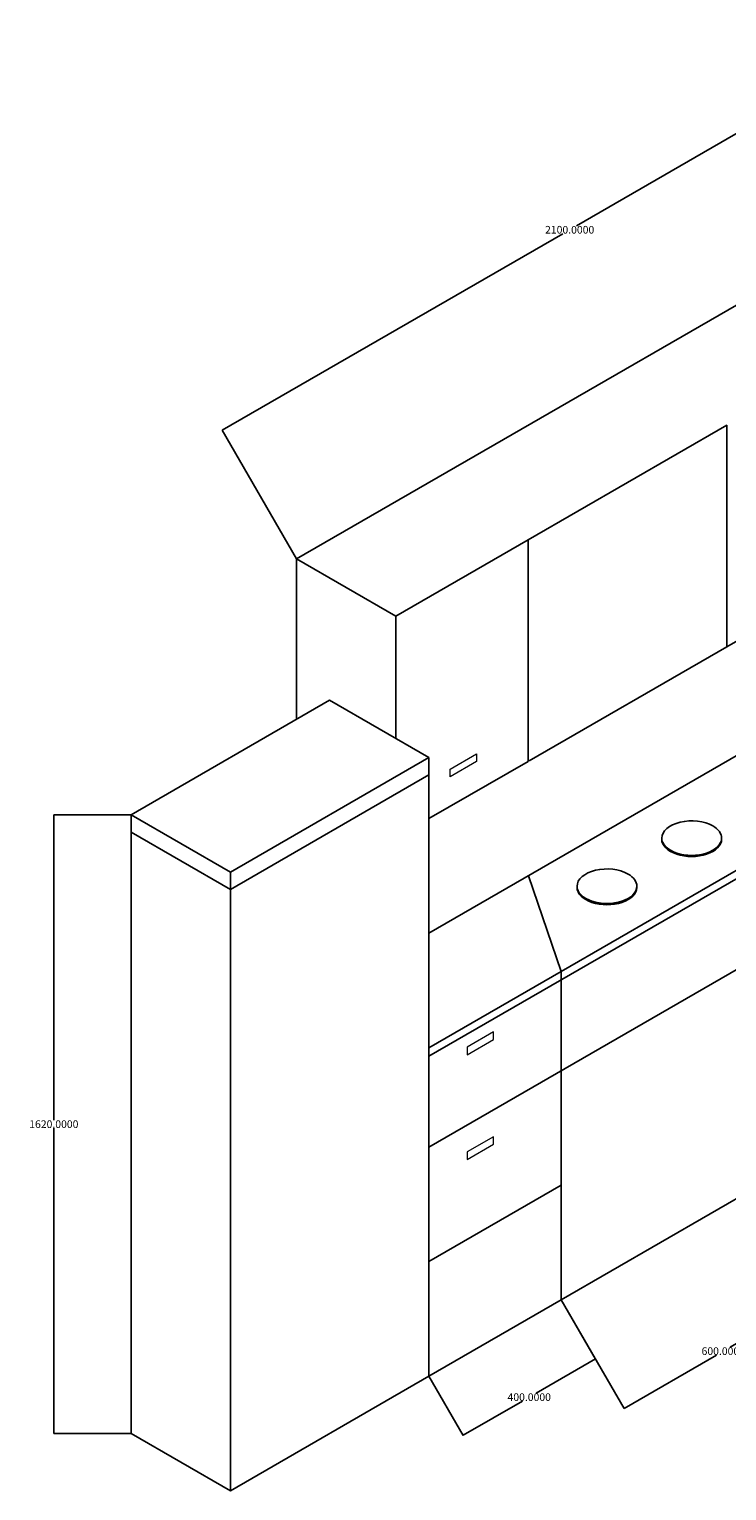
# Model space of a CAD drawing. Units: millimetres. Extents: x -886 to 3895, y -26 to 3802.
# Tile 1 of 2: x -886 to 939, y -26 to 3802. Entities that reach past the tile are written whole.
import ezdxf

# ---------------------------------------------------------------- set-up
doc = ezdxf.new("R2010")
doc.units = ezdxf.units.MM
doc.header["$MEASUREMENT"] = 0
for name, color, linetype, lineweight in [('A-ANNO-DIMS', 2, 'Continuous', 18), ('A-FURN', 7, 'Continuous', 25), ('A-FURN-HDWR', 8, 'Continuous', 18)]:
    doc.layers.add(name, color=color, linetype=linetype, lineweight=lineweight)
doc.styles.get("Standard").update_dxf_attribs({"font": 'arial.ttf'})
doc.dimstyles.get("Standard").update_dxf_attribs({"dimtxt": 0.18, "dimasz": 0.18, "dimexe": 0.18, "dimexo": 0.0625, "dimgap": 0.09, "dimtad": 0, "dimtih": 1, "dimtoh": 1, "dimdec": 4, "dimzin": 0, "dimdsep": 46, "dimtxsty": 'Standard', "dimcen": 0.09, "dimadec": 0, "dimazin": 0, "dimtfac": 1, "dimtdec": 4, "dimtofl": 0, "dimtmove": 0, "dimatfit": 3, "dimfxl": 1, "dimtolj": 1, "dimtzin": 0, "dimarcsym": 0})

# ---------------------------------------------------------------- blocks, each defined once
blk = doc.blocks.new('*D1')
at = {"layer": 'A-ANNO-DIMS', "color": 0, "lineweight": -2, "transparency": 16777216}
for p, q in [((-619.5, 1744.3), (-821.8, 1744.3)), ((-821.6, 1744.1), (-821.6, 944.6)), ((-821.6, 124.5), (-821.6, 924)), ((-619.5, 124.3), (-821.8, 124.3))]:
    blk.add_line(p, q, dxfattribs=at)
at = {"layer": 'A-ANNO-DIMS', "color": 0, "transparency": 16777216}
for points in [[(-821.6, 1744.1), (-821.5, 1744.1), (-821.6, 1744.3)], [(-821.6, 124.5), (-821.5, 124.5), (-821.6, 124.3)]]:
    blk.add_solid(points, dxfattribs=at)
at = {"layer": 'Defpoints', "color": 0, "transparency": 16777216}
for p in [(-821.6, 1744.3), (-619.5, 1744.3), (-619.5, 124.3)]:
    blk.add_point(p, dxfattribs=at)
at = {"layer": 'A-ANNO-DIMS', "color": 0, "transparency": 16777216, "insert": (-821.6, 934.3), "char_height": 20, "attachment_point": 5}
blk.add_mtext('\\A1;1620.0000', dxfattribs=at)
blk = doc.blocks.new('*D7')
at = {"layer": 'A-ANNO-DIMS', "color": 0, "lineweight": -2, "transparency": 16777216}
for p, q in [((1437.4, 3801.3), (546.1, 3286.7)), ((1632.2, 3464.3), (1437.5, 3801.5)), ((-380.9, 2751.4), (510.4, 3266.1)), ((-186.5, 2414.3), (-381.2, 2751.5))]:
    blk.add_line(p, q, dxfattribs=at)
at = {"layer": 'A-ANNO-DIMS', "color": 0, "transparency": 16777216}
for points in [[(1437.4, 3801.3), (1437.5, 3801.2), (1437.6, 3801.4)], [(-380.9, 2751.5), (-380.9, 2751.4), (-381.1, 2751.4)]]:
    blk.add_solid(points, dxfattribs=at)
at = {"layer": 'Defpoints', "color": 0, "transparency": 16777216}
for p in [(1632.2, 3464.3), (-381.1, 2751.4), (-186.4, 2414.3)]:
    blk.add_point(p, dxfattribs=at)
at = {"layer": 'A-ANNO-DIMS', "color": 0, "transparency": 16777216, "insert": (528.3, 3276.4), "char_height": 20, "attachment_point": 5}
blk.add_mtext('\\A1;2100.0000', dxfattribs=at)
blk = doc.blocks.new('*D8')
at = {"layer": 'A-ANNO-DIMS', "color": 0, "lineweight": -2, "transparency": 16777216}
for p, q in [((506.4, 474.2), (595.8, 319.3)), ((595.6, 319.4), (440.4, 229.8)), ((160, 274.2), (249.4, 119.3)), ((249.5, 119.6), (404.7, 209.2))]:
    blk.add_line(p, q, dxfattribs=at)
at = {"layer": 'A-ANNO-DIMS', "color": 0, "transparency": 16777216}
for points in [[(595.6, 319.4), (595.6, 319.3), (595.8, 319.5)], [(249.5, 119.6), (249.5, 119.5), (249.3, 119.5)]]:
    blk.add_solid(points, dxfattribs=at)
at = {"layer": 'Defpoints', "color": 0, "transparency": 16777216}
for p in [(506.4, 474.3), (595.8, 319.5), (160, 274.3)]:
    blk.add_point(p, dxfattribs=at)
at = {"layer": 'A-ANNO-DIMS', "color": 0, "transparency": 16777216, "insert": (422.5, 219.5), "char_height": 20, "attachment_point": 5}
blk.add_mtext('\\A1;400.0000', dxfattribs=at)
blk = doc.blocks.new('*D9')
at = {"layer": 'A-ANNO-DIMS', "color": 0, "lineweight": -2, "transparency": 16777216}
for p, q in [((1026, 774.2), (1190.2, 489.9)), ((506.4, 474.2), (670.6, 189.9)), ((1189.9, 489.9), (948.1, 350.3)), ((670.6, 190.1), (912.4, 329.7))]:
    blk.add_line(p, q, dxfattribs=at)
at = {"layer": 'A-ANNO-DIMS', "color": 0, "transparency": 16777216}
for points in [[(1189.9, 490), (1190, 489.9), (1190.1, 490)], [(670.6, 190.1), (670.7, 190.1), (670.5, 190)]]:
    blk.add_solid(points, dxfattribs=at)
at = {"layer": 'Defpoints', "color": 0, "transparency": 16777216}
for p in [(1026, 774.3), (506.4, 474.3), (1190.1, 490)]:
    blk.add_point(p, dxfattribs=at)
at = {"layer": 'A-ANNO-DIMS', "color": 0, "transparency": 16777216, "insert": (930.3, 340), "char_height": 20, "attachment_point": 5}
blk.add_mtext('\\A1;600.0000', dxfattribs=at)
blk = doc.blocks.new('CAB-HANDLE-A')
blk.add_lwpolyline([(69.3, 0), (69.3, 20), (0, 60), (0, 40)], close=True)
blk = doc.blocks.new('CAB-HANDLE-B')
blk.add_lwpolyline([(69.3, 40), (69.3, 60), (0, 20), (0, 0)], close=True)

msp = doc.modelspace()

# ---------------------------------------------------------------- linework, layer by layer
at = {"layer": 'A-FURN'}
for p, q in [((73.36231, 1944.27279), (73.36231, 2264.27279)), ((422.36925, 1885.775), (939.38642, 2184.275)), ((769.20405, 1680.275), (769.20405, 1683.275)), ((925.97139, 1680.275), (925.97139, 1683.275)), ((547.50155, 1554.275), (547.50155, 1557.275)), ((704.26889, 1554.275), (704.26889, 1557.275)), ((159.96485, 574.27279), (506.37498, 774.27277))]:
    msp.add_line(p, q, dxfattribs=at)
for points in [[(3624.06646, 2614.27279), (2238.42582, 3414.27279), (1892.01566, 3614.27279), (1632.20803, 3464.27279), (-186.44531, 2414.27279)], [(2411.6309, 2434.27279), (1892.01566, 2734.27279), (1372.40041, 2434.27279), (939.38771, 2184.27279), (939.38771, 2764.27279), (419.77247, 2464.27279), (73.36231, 2264.27279), (-186.44531, 2414.27279), (-186.44531, 1994.27279)], [(159.96485, 1134.27286), (159.96485, 1434.27286), (1978.6182, 2484.27286), (2238.42582, 2334.27286), (3624.06646, 1534.27286)], [(419.77247, 2464.27279), (419.77247, 1884.27279), (159.96485, 1734.27279)], [(159.96485, 1111.93531), (1978.6182, 2161.93531), (3364.25884, 1361.93531)], [(1025.99022, 1634.27284), (506.37498, 1334.27284), (506.37498, 474.27284), (159.96485, 274.27279), (159.96485, 1894.27279), (-99.84277, 2044.27279), (-619.45802, 1744.27279), (-619.45802, 124.27279), (-359.65039, -25.72721), (-359.65039, 1594.27279)], [(3364.25884, 1124.27279), (1978.6182, 1924.27279), (159.96485, 874.27279)], [(-619.45802, 1744.27279), (-359.65039, 1594.27279), (159.96485, 1894.27279)], [(-619.45802, 1699.08214), (-359.65039, 1549.08214), (159.96485, 1849.08214)], [(420.75707, 1584.84132), (506.37498, 1334.27284), (159.96482, 1134.27284)], [(-359.65039, -25.72721), (159.96485, 274.27279), (506.37501, 474.27279), (1025.99025, 774.27279), (1978.6182, 1324.27279)]]:
    msp.add_lwpolyline(points, dxfattribs=at)
for centre, start_param, end_param in [((847.58772, 1683.275), 0.7853981634, 3.1415926536), ((847.58772, 1683.275), 0, 0.7853981634), ((847.58772, 1683.275), 3.1415926536, 6.2831853072), ((847.58772, 1680.275), 3.1084409511, 3.1415926536), ((847.58772, 1680.275), 3.1415926536, 6.2831853072), ((847.58772, 1680.275), 0, 0.0331517025), ((625.88522, 1557.275), 0.7853981634, 3.1415926536), ((625.88522, 1557.275), 0, 0.7853981634), ((625.88522, 1557.275), 3.1415926536, 6.2831853072), ((625.88522, 1554.275), 3.1084409511, 3.1415926536), ((625.88522, 1554.275), 3.1415926536, 6.2831853072), ((625.88522, 1554.275), 0, 0.0331517025)]:
    msp.add_ellipse(centre, major_axis=(78.38367, 0), ratio=0.5773502692, start_param=start_param, end_param=end_param, dxfattribs=at)

# ---------------------------------------------------------------- block references
at = {"layer": 'A-FURN-HDWR', "extrusion": (0, 0, -1), "zscale": -1, "rotation": 180}
msp.add_blockref('CAB-HANDLE-A', (-215.30381, 1903.8946), dxfattribs=at)
at = {"layer": 'A-FURN-HDWR'}
for p in [(259.67283, 1116.25572), (259.67283, 841.47545)]:
    msp.add_blockref('CAB-HANDLE-B', p, dxfattribs=at)

# ---------------------------------------------------------------- dimensions: what is measured, and where the dimension line sits
at = {"layer": 'A-ANNO-DIMS'}
for p1, p2, distance, picture, middle in [((1632.20803, 3464.27279), (-186.44531, 2414.27279), -389.2306, '*D7', (528.26606, 3276.35638)), ((506.37498, 474.27284), (1025.99025, 774.27279), -328.21158, '*D9', (930.28837, 340.03324)), ((159.96485, 274.27279), (506.37501, 474.27279), -178.75749, '*D8', (422.54868, 219.46426))]:
    dim = msp.add_aligned_dim(p1=p1, p2=p2, distance=distance, dimstyle='Standard', override={"dimtxt": 20, "dimclrd": 0, "dimclre": 0, "dimclrt": 0}, dxfattribs=at)
    dim.commit()
    dim.dimension.update_dxf_attribs({"geometry": picture, "text_midpoint": middle})
dim = msp.add_linear_dim(base=(-821.57216, 1744.27279), p1=(-619.45802, 124.27279), p2=(-619.45802, 1744.27279), angle=90, dimstyle='Standard', override={"dimtxt": 20, "dimclrd": 0, "dimclre": 0, "dimclrt": 0}, dxfattribs=at)
dim.commit()
dim.dimension.update_dxf_attribs({"geometry": '*D1', "text_midpoint": (-821.57216, 934.27279)})

doc.saveas('drawing.dxf')
